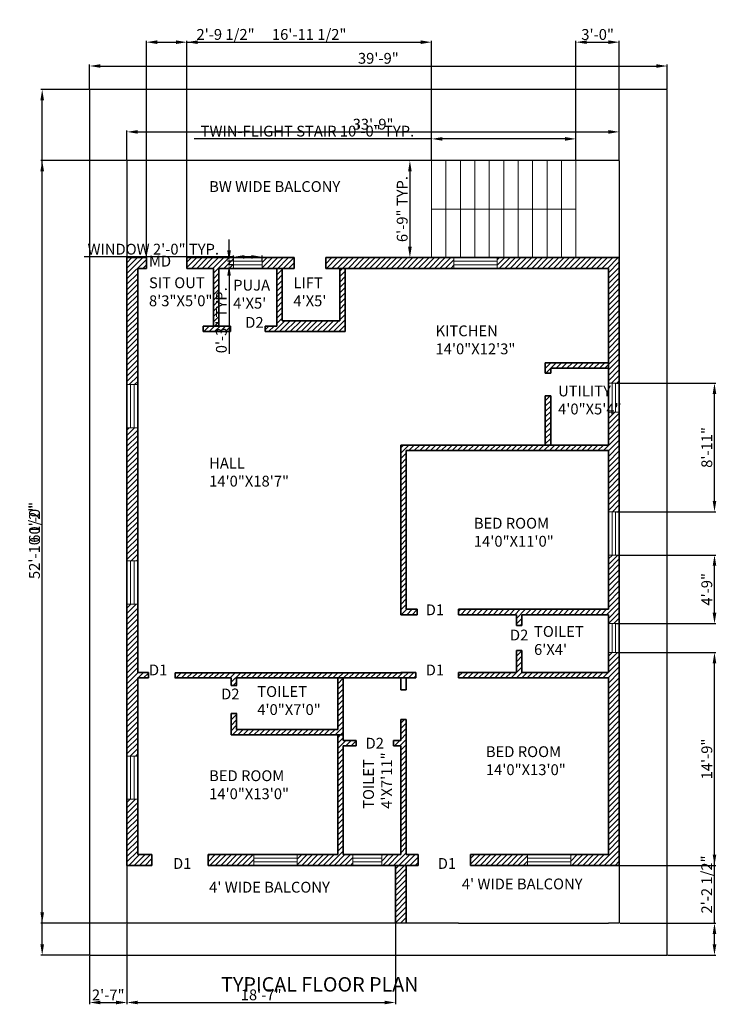
# Model space of a CAD drawing. Units: inches. Extents: x 9573 to 10767, y 4927 to 5746.
# Tile 2 of 2: x 10182 to 10767, y 4927 to 5746. Entities that reach past the tile are written whole.
import ezdxf

# ---------------------------------------------------------------- set-up
doc = ezdxf.new("R2010")
doc.units = ezdxf.units.IN
for name, color, linetype, lineweight in [('A-ANNO-DIMS', 2, 'Continuous', 18), ('A-ANNO-TEXT', 7, 'Continuous', 25), ('A-AREA-IDEN', 7, 'Continuous', 18), ('A-DOOR-IDEN', 3, 'Continuous', 18), ('A-FLOR-BALC', 7, 'Continuous', 25), ('A-FLOR-STRS', 7, 'Continuous', 18), ('A-GLAZ', 4, 'Continuous', 18), ('A-WALL', 7, 'Continuous', 35), ('A-WALL-PATT', 252, 'Continuous', 13), ('C-PROP', 8, 'Continuous', 25)]:
    doc.layers.add(name, color=color, linetype=linetype, lineweight=lineweight)
doc.styles.get("Standard").update_dxf_attribs({"font": 'arial.ttf'})
doc.dimstyles.new('ISO-25', dxfattribs={"dimtxt": 9, "dimasz": 9, "dimexe": 1.25, "dimexo": 0.625, "dimtad": 1, "dimdec": 1, "dimrnd": 9, "dimlunit": 3, "dimtxsty": 'Standard', "dimcen": 2.5, "dimadec": 0, "dimazin": 0, "dimtfac": 1, "dimtdec": 1, "dimtmove": 0, "dimatfit": 3, "dimfxl": 1, "dimarcsym": 0})
pattern_1 = [(45, (609.373, 0), (-2.245064, 2.245064), [])]

# ---------------------------------------------------------------- blocks, each defined once
blk = doc.blocks.new('*D3')
at = {"layer": 'A-ANNO-DIMS', "color": 0, "lineweight": -2, "transparency": 16777216}
for p, q in [((10271.02, 5629.81), (10271.02, 5654.25)), ((10280.02, 5653), (10671.21, 5653)), ((10680.21, 5629.81), (10680.21, 5654.25))]:
    blk.add_line(p, q, dxfattribs=at)
at = {"layer": 'A-ANNO-DIMS', "color": 0, "transparency": 16777216}
for points in [[(10280.02, 5654.5), (10280.02, 5651.5), (10271.02, 5653)], [(10671.21, 5654.5), (10671.21, 5651.5), (10680.21, 5653)]]:
    blk.add_solid(points, dxfattribs=at)
at = {"layer": 'Defpoints', "color": 0, "transparency": 16777216}
for p in [(10680.21, 5653), (10271.02, 5629.18), (10680.21, 5629.18)]:
    blk.add_point(p, dxfattribs=at)
at = {"layer": 'A-ANNO-DIMS', "color": 0, "transparency": 16777216, "insert": (10475.62, 5658.23), "char_height": 9, "attachment_point": 5}
blk.add_mtext('33\'-9"', dxfattribs=at)
blk = doc.blocks.new('*D4')
at = {"layer": 'A-ANNO-DIMS', "color": 0, "lineweight": -2, "transparency": 16777216}
for p, q in [((10240, 5688.89), (10240, 5709.04)), ((10249, 5707.79), (10711, 5707.79)), ((10720, 5688.89), (10720, 5709.04))]:
    blk.add_line(p, q, dxfattribs=at)
at = {"layer": 'A-ANNO-DIMS', "color": 0, "transparency": 16777216}
for points in [[(10249, 5709.29), (10249, 5706.29), (10240, 5707.79)], [(10711, 5709.29), (10711, 5706.29), (10720, 5707.79)]]:
    blk.add_solid(points, dxfattribs=at)
at = {"layer": 'Defpoints', "color": 0, "transparency": 16777216}
for p in [(10720, 5707.79), (10240, 5688.26), (10720, 5688.26)]:
    blk.add_point(p, dxfattribs=at)
at = {"layer": 'A-ANNO-DIMS', "color": 0, "transparency": 16777216, "insert": (10480, 5713.01), "char_height": 9, "attachment_point": 5}
blk.add_mtext('39\'-9"', dxfattribs=at)
blk = doc.blocks.new('GLAZ-36IN')
for p, q in [((0, 3), (36, 3)), ((0, 0), (36, 0))]:
    blk.add_line(p, q)
blk = doc.blocks.new('GLAZ-24IN')
for p, q in [((0, 3), (24, 3)), ((0, 0), (24, 0))]:
    blk.add_line(p, q)
blk = doc.blocks.new('STAIR-TWIN-FLIGHT')
for p, q in [((0, 80.77), (0, 0)), ((12, 80.77), (12, 0)), ((24, 80.77), (24, 0)), ((36, 80.77), (36, 0)), ((48, 80.77), (48, 0)), ((60, 80.77), (60, 0)), ((72, 80.77), (72, 0)), ((84, 80.77), (84, 0)), ((96, 80.77), (96, 0)), ((108, 80.77), (108, 0)), ((120, 80.77), (120, 0)), ((0, 40.39), (120, 40.39))]:
    blk.add_line(p, q)
blk = doc.blocks.new('*D10')
at = {"layer": 'A-ANNO-DIMS', "color": 0, "lineweight": -2, "transparency": 16777216}
for p, q in [((10359.53, 5549.01), (10235.39, 5549.01)), ((10359.53, 5546.03), (10359.53, 5550.26)), ((10374.53, 5549.01), (10368.53, 5549.01)), ((10383.53, 5546.03), (10383.53, 5550.26))]:
    blk.add_line(p, q, dxfattribs=at)
at = {"layer": 'A-ANNO-DIMS', "color": 0, "transparency": 16777216}
for points in [[(10368.53, 5550.51), (10368.53, 5547.51), (10359.53, 5549.01)], [(10374.53, 5550.51), (10374.53, 5547.51), (10383.53, 5549.01)]]:
    blk.add_solid(points, dxfattribs=at)
at = {"layer": 'Defpoints', "color": 0, "transparency": 16777216}
for p in [(10359.53, 5549.01), (10359.53, 5545.41), (10383.53, 5545.41)]:
    blk.add_point(p, dxfattribs=at)
at = {"layer": 'A-ANNO-DIMS', "color": 0, "transparency": 16777216, "insert": (10292.96, 5554.29), "char_height": 9, "attachment_point": 5}
blk.add_mtext('WINDOW 2\'-0" TYP.', dxfattribs=at)
blk = doc.blocks.new('*D11')
at = {"layer": 'A-ANNO-DIMS', "color": 0, "lineweight": -2, "transparency": 16777216}
for p, q in [((10355.93, 5554.41), (10355.93, 5563.41)), ((10358.9, 5545.41), (10354.68, 5545.41)), ((10355.93, 5545.41), (10355.93, 5542.41)), ((10358.9, 5542.41), (10354.68, 5542.41)), ((10355.93, 5533.41), (10355.93, 5468.3))]:
    blk.add_line(p, q, dxfattribs=at)
at = {"layer": 'A-ANNO-DIMS', "color": 0, "transparency": 16777216}
for points in [[(10354.43, 5554.41), (10357.43, 5554.41), (10355.93, 5545.41)], [(10354.43, 5533.41), (10357.43, 5533.41), (10355.93, 5542.41)]]:
    blk.add_solid(points, dxfattribs=at)
at = {"layer": 'Defpoints', "color": 0, "transparency": 16777216}
for p in [(10359.53, 5545.41), (10355.93, 5542.41), (10359.53, 5542.41)]:
    blk.add_point(p, dxfattribs=at)
at = {"layer": 'A-ANNO-DIMS', "color": 0, "transparency": 16777216, "insert": (10350.7, 5496.35), "char_height": 9, "attachment_point": 5, "rotation": 90}
blk.add_mtext('0\'-3" TYP.', dxfattribs=at)
blk = doc.blocks.new('*D12')
at = {"layer": 'A-ANNO-DIMS', "color": 0, "lineweight": -2, "transparency": 16777216}
for p, q in [((10524.21, 5647.18), (10326.86, 5647.18)), ((10524.21, 5629.81), (10524.21, 5648.43)), ((10635.21, 5647.18), (10533.21, 5647.18)), ((10644.21, 5629.81), (10644.21, 5648.43))]:
    blk.add_line(p, q, dxfattribs=at)
at = {"layer": 'A-ANNO-DIMS', "color": 0, "transparency": 16777216}
for points in [[(10533.21, 5648.68), (10533.21, 5645.68), (10524.21, 5647.18)], [(10635.21, 5648.68), (10635.21, 5645.68), (10644.21, 5647.18)]]:
    blk.add_solid(points, dxfattribs=at)
at = {"layer": 'Defpoints', "color": 0, "transparency": 16777216}
for p in [(10524.21, 5647.18), (10524.21, 5629.18), (10644.21, 5629.18)]:
    blk.add_point(p, dxfattribs=at)
at = {"layer": 'A-ANNO-DIMS', "color": 0, "transparency": 16777216, "insert": (10421.04, 5652.46), "char_height": 9, "attachment_point": 5}
blk.add_mtext('TWIN-FLIGHT STAIR 10\'-0" TYP.', dxfattribs=at)
blk = doc.blocks.new('*D13')
at = {"layer": 'A-ANNO-DIMS', "color": 0, "lineweight": -2, "transparency": 16777216}
for p, q in [((10523.59, 5629.18), (10504.96, 5629.18)), ((10506.21, 5620.18), (10506.21, 5557.41)), ((10523.59, 5548.41), (10504.96, 5548.41))]:
    blk.add_line(p, q, dxfattribs=at)
at = {"layer": 'A-ANNO-DIMS', "color": 0, "transparency": 16777216}
for points in [[(10504.71, 5620.18), (10507.71, 5620.18), (10506.21, 5629.18)], [(10504.71, 5557.41), (10507.71, 5557.41), (10506.21, 5548.41)]]:
    blk.add_solid(points, dxfattribs=at)
at = {"layer": 'Defpoints', "color": 0, "transparency": 16777216}
for p in [(10524.21, 5629.18), (10506.21, 5548.41), (10524.21, 5548.41)]:
    blk.add_point(p, dxfattribs=at)
at = {"layer": 'A-ANNO-DIMS', "color": 0, "transparency": 16777216, "insert": (10500.99, 5588.8), "char_height": 9, "attachment_point": 5, "rotation": 90}
blk.add_mtext('6\'-9" TYP.', dxfattribs=at)
blk = doc.blocks.new('*D18')
at = {"layer": 'A-ANNO-DIMS', "color": 0, "lineweight": -2, "transparency": 16777216}
for p, q in [((10270.39, 5629.18), (10199.4, 5629.18)), ((10200.65, 5003.91), (10200.65, 5620.18)), ((10270.39, 4994.91), (10199.4, 4994.91))]:
    blk.add_line(p, q, dxfattribs=at)
at = {"layer": 'A-ANNO-DIMS', "color": 0, "transparency": 16777216}
for points in [[(10199.15, 5620.18), (10202.15, 5620.18), (10200.65, 5629.18)], [(10199.15, 5003.91), (10202.15, 5003.91), (10200.65, 4994.91)]]:
    blk.add_solid(points, dxfattribs=at)
at = {"layer": 'Defpoints', "color": 0, "transparency": 16777216}
for p in [(10200.65, 5629.18), (10271.02, 5629.18), (10271.02, 4994.91)]:
    blk.add_point(p, dxfattribs=at)
at = {"layer": 'A-ANNO-DIMS', "color": 0, "transparency": 16777216, "insert": (10195.37, 5312.05), "char_height": 9, "attachment_point": 5, "rotation": 90}
blk.add_mtext('52\'-10 1/2"', dxfattribs=at)
blk = doc.blocks.new('*D19')
at = {"layer": 'A-ANNO-DIMS', "color": 0, "lineweight": -2, "transparency": 16777216}
for p, q in [((10239.38, 5688.26), (10199.4, 5688.26)), ((10200.65, 4977.26), (10200.65, 5679.26)), ((10239.38, 4968.26), (10199.4, 4968.26))]:
    blk.add_line(p, q, dxfattribs=at)
at = {"layer": 'A-ANNO-DIMS', "color": 0, "transparency": 16777216}
for points in [[(10199.15, 5679.26), (10202.15, 5679.26), (10200.65, 5688.26)], [(10199.15, 4977.26), (10202.15, 4977.26), (10200.65, 4968.26)]]:
    blk.add_solid(points, dxfattribs=at)
at = {"layer": 'Defpoints', "color": 0, "transparency": 16777216}
for p in [(10200.65, 5688.26), (10240, 5688.26), (10240, 4968.26)]:
    blk.add_point(p, dxfattribs=at)
at = {"layer": 'A-ANNO-DIMS', "color": 0, "transparency": 16777216, "insert": (10195.43, 5328.26), "char_height": 9, "attachment_point": 5, "rotation": 90}
blk.add_mtext('60\'-0"', dxfattribs=at)
blk = doc.blocks.new('*D20')
at = {"layer": 'A-ANNO-DIMS', "color": 0, "lineweight": -2, "transparency": 16777216}
for p, q in [((10271.02, 4994.28), (10271.02, 4927.66)), ((10240, 4967.64), (10240, 4927.66)), ((10249, 4928.91), (10262.02, 4928.91))]:
    blk.add_line(p, q, dxfattribs=at)
at = {"layer": 'A-ANNO-DIMS', "color": 0, "transparency": 16777216}
for points in [[(10249, 4930.41), (10249, 4927.41), (10240, 4928.91)], [(10262.02, 4930.41), (10262.02, 4927.41), (10271.02, 4928.91)]]:
    blk.add_solid(points, dxfattribs=at)
at = {"layer": 'Defpoints', "color": 0, "transparency": 16777216}
for p in [(10271.02, 4994.91), (10240, 4968.26), (10271.02, 4928.91)]:
    blk.add_point(p, dxfattribs=at)
at = {"layer": 'A-ANNO-DIMS', "color": 0, "transparency": 16777216, "insert": (10255.51, 4934.06), "char_height": 9, "attachment_point": 5}
blk.add_mtext('2\'-7"', dxfattribs=at)
blk = doc.blocks.new('*D21')
at = {"layer": 'A-ANNO-DIMS', "color": 0, "lineweight": -2, "transparency": 16777216}
for p, q in [((10759.35, 4994.91), (10759.35, 5050.21)), ((10680.84, 4994.91), (10760.6, 4994.91)), ((10759.35, 4977.26), (10759.35, 4985.91)), ((10720.62, 4968.26), (10760.6, 4968.26))]:
    blk.add_line(p, q, dxfattribs=at)
at = {"layer": 'A-ANNO-DIMS', "color": 0, "transparency": 16777216}
for points in [[(10757.85, 4985.91), (10760.85, 4985.91), (10759.35, 4994.91)], [(10757.85, 4977.26), (10760.85, 4977.26), (10759.35, 4968.26)]]:
    blk.add_solid(points, dxfattribs=at)
at = {"layer": 'Defpoints', "color": 0, "transparency": 16777216}
for p in [(10680.21, 4994.91), (10759.35, 4994.91), (10720, 4968.26)]:
    blk.add_point(p, dxfattribs=at)
at = {"layer": 'A-ANNO-DIMS', "color": 0, "transparency": 16777216, "insert": (10754.07, 5027.06), "char_height": 9, "attachment_point": 5, "rotation": 90}
blk.add_mtext('2\'-2 1/2"', dxfattribs=at)
blk = doc.blocks.new('*D23')
at = {"layer": 'A-ANNO-DIMS', "color": 0, "lineweight": -2, "transparency": 16777216}
for p, q in [((10644.21, 5629.81), (10644.21, 5728.86)), ((10653.21, 5727.61), (10671.21, 5727.61)), ((10680.21, 5629.81), (10680.21, 5728.86))]:
    blk.add_line(p, q, dxfattribs=at)
at = {"layer": 'A-ANNO-DIMS', "color": 0, "transparency": 16777216}
for points in [[(10653.21, 5729.11), (10653.21, 5726.11), (10644.21, 5727.61)], [(10671.21, 5729.11), (10671.21, 5726.11), (10680.21, 5727.61)]]:
    blk.add_solid(points, dxfattribs=at)
at = {"layer": 'Defpoints', "color": 0, "transparency": 16777216}
for p in [(10680.21, 5727.61), (10644.21, 5629.18), (10680.21, 5629.18)]:
    blk.add_point(p, dxfattribs=at)
at = {"layer": 'A-ANNO-DIMS', "color": 0, "transparency": 16777216, "insert": (10662.21, 5732.83), "char_height": 9, "attachment_point": 5}
blk.add_mtext('3\'-0"', dxfattribs=at)
blk = doc.blocks.new('*D26')
at = {"layer": 'A-ANNO-DIMS', "color": 0, "lineweight": -2, "transparency": 16777216}
for p, q in [((10287.2, 5549.03), (10287.2, 5728.86)), ((10296.2, 5727.61), (10311.84, 5727.61)), ((10320.84, 5549.03), (10320.84, 5728.86)), ((10320.84, 5727.61), (10376.14, 5727.61))]:
    blk.add_line(p, q, dxfattribs=at)
at = {"layer": 'A-ANNO-DIMS', "color": 0, "transparency": 16777216}
for points in [[(10296.2, 5729.11), (10296.2, 5726.11), (10287.2, 5727.61)], [(10311.84, 5729.11), (10311.84, 5726.11), (10320.84, 5727.61)]]:
    blk.add_solid(points, dxfattribs=at)
at = {"layer": 'Defpoints', "color": 0, "transparency": 16777216}
for p in [(10320.84, 5727.61), (10287.2, 5548.41), (10320.84, 5548.41)]:
    blk.add_point(p, dxfattribs=at)
at = {"layer": 'A-ANNO-DIMS', "color": 0, "transparency": 16777216, "insert": (10352.99, 5732.89), "char_height": 9, "attachment_point": 5}
blk.add_mtext('2\'-9 1/2"', dxfattribs=at)
blk = doc.blocks.new('*D27')
at = {"layer": 'A-ANNO-DIMS', "color": 0, "lineweight": -2, "transparency": 16777216}
for p, q in [((10320.84, 5549.03), (10320.84, 5728.86)), ((10329.84, 5727.61), (10515.21, 5727.61)), ((10524.21, 5629.81), (10524.21, 5728.86))]:
    blk.add_line(p, q, dxfattribs=at)
at = {"layer": 'A-ANNO-DIMS', "color": 0, "transparency": 16777216}
for points in [[(10329.84, 5729.11), (10329.84, 5726.11), (10320.84, 5727.61)], [(10515.21, 5729.11), (10515.21, 5726.11), (10524.21, 5727.61)]]:
    blk.add_solid(points, dxfattribs=at)
at = {"layer": 'Defpoints', "color": 0, "transparency": 16777216}
for p in [(10524.21, 5727.61), (10524.21, 5629.18), (10320.84, 5548.41)]:
    blk.add_point(p, dxfattribs=at)
at = {"layer": 'A-ANNO-DIMS', "color": 0, "transparency": 16777216, "insert": (10422.52, 5732.89), "char_height": 9, "attachment_point": 5}
blk.add_mtext('16\'-11 1/2"', dxfattribs=at)
blk = doc.blocks.new('*D31')
at = {"layer": 'A-ANNO-DIMS', "color": 0, "lineweight": -2, "transparency": 16777216}
for p, q in [((10677.84, 5220), (10760.6, 5220)), ((10759.35, 5051.91), (10759.35, 5211)), ((10680.84, 5042.91), (10760.6, 5042.91))]:
    blk.add_line(p, q, dxfattribs=at)
at = {"layer": 'A-ANNO-DIMS', "color": 0, "transparency": 16777216}
for points in [[(10757.85, 5211), (10760.85, 5211), (10759.35, 5220)], [(10757.85, 5051.91), (10760.85, 5051.91), (10759.35, 5042.91)]]:
    blk.add_solid(points, dxfattribs=at)
at = {"layer": 'Defpoints', "color": 0, "transparency": 16777216}
for p in [(10677.21, 5220), (10759.35, 5220), (10680.21, 5042.91)]:
    blk.add_point(p, dxfattribs=at)
at = {"layer": 'A-ANNO-DIMS', "color": 0, "transparency": 16777216, "insert": (10754.13, 5131.45), "char_height": 9, "attachment_point": 5, "rotation": 90}
blk.add_mtext('14\'-9"', dxfattribs=at)
blk = doc.blocks.new('*D32')
at = {"layer": 'A-ANNO-DIMS', "color": 0, "lineweight": -2, "transparency": 16777216}
for p, q in [((10677.84, 5301.09), (10760.6, 5301.09)), ((10759.35, 5253), (10759.35, 5292.09)), ((10677.84, 5244), (10760.6, 5244))]:
    blk.add_line(p, q, dxfattribs=at)
at = {"layer": 'A-ANNO-DIMS', "color": 0, "transparency": 16777216}
for points in [[(10757.85, 5292.09), (10760.85, 5292.09), (10759.35, 5301.09)], [(10757.85, 5253), (10760.85, 5253), (10759.35, 5244)]]:
    blk.add_solid(points, dxfattribs=at)
at = {"layer": 'Defpoints', "color": 0, "transparency": 16777216}
for p in [(10677.21, 5301.09), (10759.35, 5301.09), (10677.21, 5244)]:
    blk.add_point(p, dxfattribs=at)
at = {"layer": 'A-ANNO-DIMS', "color": 0, "transparency": 16777216, "insert": (10754.13, 5272.55), "char_height": 9, "attachment_point": 5, "rotation": 90}
blk.add_mtext('4\'-9"', dxfattribs=at)
blk = doc.blocks.new('*D33')
at = {"layer": 'A-ANNO-DIMS', "color": 0, "lineweight": -2, "transparency": 16777216}
for p, q in [((10677.84, 5444), (10760.6, 5444)), ((10759.35, 5346.09), (10759.35, 5435)), ((10677.84, 5337.09), (10760.6, 5337.09))]:
    blk.add_line(p, q, dxfattribs=at)
at = {"layer": 'A-ANNO-DIMS', "color": 0, "transparency": 16777216}
for points in [[(10757.85, 5435), (10760.85, 5435), (10759.35, 5444)], [(10757.85, 5346.09), (10760.85, 5346.09), (10759.35, 5337.09)]]:
    blk.add_solid(points, dxfattribs=at)
at = {"layer": 'Defpoints', "color": 0, "transparency": 16777216}
for p in [(10677.21, 5444), (10759.35, 5444), (10677.21, 5337.09)]:
    blk.add_point(p, dxfattribs=at)
at = {"layer": 'A-ANNO-DIMS', "color": 0, "transparency": 16777216, "insert": (10754.13, 5390.55), "char_height": 9, "attachment_point": 5, "rotation": 90}
blk.add_mtext('8\'-11"', dxfattribs=at)
blk = doc.blocks.new('*D35')
at = {"layer": 'A-ANNO-DIMS', "color": 0, "lineweight": -2, "transparency": 16777216}
for p, q in [((10271.02, 4994.28), (10271.02, 4927.66)), ((10494.21, 4994.28), (10494.21, 4927.66)), ((10280.02, 4928.91), (10485.21, 4928.91))]:
    blk.add_line(p, q, dxfattribs=at)
at = {"layer": 'A-ANNO-DIMS', "color": 0, "transparency": 16777216}
for points in [[(10280.02, 4930.41), (10280.02, 4927.41), (10271.02, 4928.91)], [(10485.21, 4930.41), (10485.21, 4927.41), (10494.21, 4928.91)]]:
    blk.add_solid(points, dxfattribs=at)
at = {"layer": 'Defpoints', "color": 0, "transparency": 16777216}
for p in [(10271.02, 4994.91), (10494.21, 4994.91), (10494.21, 4928.91)]:
    blk.add_point(p, dxfattribs=at)
at = {"layer": 'A-ANNO-DIMS', "color": 0, "transparency": 16777216, "insert": (10382.62, 4934.13), "char_height": 9, "attachment_point": 5}
blk.add_mtext('18\'-7"', dxfattribs=at)

msp = doc.modelspace()

# ---------------------------------------------------------------- hatches: boundary and pattern name
at = {"layer": 'A-WALL-PATT'}
h = msp.add_hatch(dxfattribs=at)
h.set_pattern_fill('ANSI31', color=256)
h.set_pattern_definition(pattern_1)
h.paths.add_polyline_path([(10409.99, 5548.41), (10383.53, 5548.41), (10383.53, 5539.41), (10409.99, 5539.41)])
h.paths.add_polyline_path([(10400.02, 5539.41), (10395.52, 5539.41), (10395.52, 5491.41), (10385.93, 5491.41), (10385.93, 5486.91), (10400.02, 5486.91), (10452.52, 5486.91), (10452.52, 5539.41), (10448.02, 5539.41), (10448.02, 5495.91), (10400.02, 5495.91)])
h.paths.add_polyline_path([(10357.22, 5491.41), (10334.5, 5491.41), (10334.5, 5486.91), (10357.22, 5486.91)])
h.paths.add_polyline_path([(10542.76, 5548.41), (10436.27, 5548.41), (10436.27, 5539.41), (10542.76, 5539.41)])
h.paths.add_polyline_path([(10680.21, 5548.41), (10578.76, 5548.41), (10578.76, 5539.41), (10671.21, 5539.41), (10671.21, 5444), (10680.21, 5444)])
h.paths.add_polyline_path([(10680.21, 5420), (10671.21, 5420), (10671.21, 5392.41), (10498.71, 5392.41), (10498.71, 5251.41), (10512.35, 5251.41), (10512.35, 5255.91), (10503.21, 5255.91), (10503.21, 5387.91), (10671.21, 5387.91), (10671.21, 5337.09), (10680.21, 5337.09)])
h.paths.add_polyline_path([(10623.21, 5433.61), (10618.71, 5433.61), (10618.71, 5392.41), (10623.21, 5392.41)])
h.paths.add_polyline_path([(10671.21, 5460.91), (10618.71, 5460.91), (10618.71, 5452.41), (10623.21, 5452.41), (10623.21, 5456.41), (10671.21, 5456.41)], flags=17)
h.paths.add_polyline_path([(10280.02, 5406.85), (10271.02, 5406.85), (10271.02, 5296.18), (10280.02, 5296.18)])
h.paths.add_polyline_path([(10280.02, 5486.91), (10280.02, 5491.41), (10280.02, 5539.41), (10287.2, 5539.41), (10287.2, 5548.41), (10271.02, 5548.41), (10271.02, 5442.85), (10280.02, 5442.85)])
h.paths.add_polyline_path([(10291.82, 5051.91), (10280.02, 5051.91), (10280.02, 5097.91), (10271.02, 5097.91), (10271.02, 5065.4), (10271.02, 5042.91), (10291.82, 5042.91)])
h.paths.add_polyline_path([(10450.71, 5198.91), (10446.21, 5198.91), (10446.21, 5155.91), (10362.21, 5155.91), (10362.21, 5169.21), (10357.71, 5169.21), (10357.71, 5151.41), (10450.71, 5151.41)])
h = msp.add_hatch(dxfattribs=at)
h.set_pattern_fill('ANSI31', color=256)
h.set_pattern_definition(pattern_1)
h.paths.add_polyline_path([(10376.44, 5051.91), (10338.48, 5051.91), (10338.48, 5042.91), (10376.44, 5042.91)])
h.paths.add_polyline_path([(10280.02, 5198.91), (10288.95, 5198.91), (10288.95, 5203.27), (10280.02, 5203.26), (10280.02, 5260.18), (10271.02, 5260.18), (10271.02, 5133.91), (10280.02, 5133.91)])
h.paths.add_polyline_path([(10458.85, 5051.91), (10450.71, 5051.91), (10450.71, 5142.41), (10461.55, 5142.41), (10461.55, 5146.91), (10450.71, 5146.91), (10450.71, 5151.41), (10446.21, 5151.41), (10446.21, 5051.91), (10412.44, 5051.91), (10412.44, 5042.91), (10458.85, 5042.91)])
h.paths.add_polyline_path([(10511.15, 5203.41), (10498.71, 5203.4), (10498.71, 5203.23), (10311.25, 5203.23), (10311.25, 5198.91), (10357.71, 5198.91), (10357.71, 5192.53), (10362.21, 5192.53), (10362.21, 5198.91), (10511.15, 5198.91)])
h.paths.add_polyline_path([(10503.21, 5164.29), (10498.71, 5164.29), (10498.71, 5146.91), (10492.55, 5146.91), (10492.55, 5142.41), (10498.71, 5142.41), (10498.71, 5051.91), (10482.85, 5051.91), (10482.85, 5042.91), (10512.97, 5042.91), (10512.97, 5051.91), (10503.21, 5051.91)])
h.paths.add_polyline_path([(10503.21, 5042.91), (10494.21, 5042.91), (10494.21, 4994.91), (10503.21, 4994.91)])
h.paths.add_polyline_path([(10603.97, 5051.91), (10556.66, 5051.91), (10556.66, 5042.91), (10603.97, 5042.91)], flags=17)
h.paths.add_polyline_path([(10680.21, 5065.4), (10680.21, 5220), (10671.21, 5220), (10671.21, 5203.41), (10599.21, 5203.41), (10599.21, 5221.8), (10594.71, 5221.8), (10594.71, 5203.41), (10546.72, 5203.41), (10546.72, 5198.91), (10671.21, 5198.91), (10671.21, 5051.91), (10639.97, 5051.91), (10639.97, 5042.91), (10671.21, 5042.91), (10680.21, 5042.91)])
h.paths.add_polyline_path([(10680.21, 5301.09), (10671.21, 5301.09), (10671.21, 5255.91), (10546.72, 5255.91), (10546.72, 5251.41), (10594.71, 5251.41), (10594.71, 5242.53), (10599.21, 5242.53), (10599.21, 5251.41), (10671.21, 5251.41), (10671.21, 5244), (10680.21, 5244)])
h.paths.add_polyline_path([(10359.53, 5548.41), (10320.84, 5548.41), (10320.84, 5539.41), (10343.02, 5539.41), (10343.02, 5491.41), (10347.52, 5491.41), (10347.52, 5539.41), (10359.53, 5539.41)])

# ---------------------------------------------------------------- linework, layer by layer
at = {"layer": 'A-FLOR-BALC'}
for p, q in [((10680.21, 5629.18), (10271.02, 5629.18)), ((10271.02, 5629.18), (10271.02, 5548.41)), ((10680.21, 5629.18), (10680.21, 5548.41)), ((10271.02, 5042.91), (10271.02, 4994.91)), ((10680.21, 5042.91), (10680.21, 4994.91)), ((10546.72, 4994.91), (10271.02, 4994.91)), ((10546.72, 4994.91), (10671.21, 4994.91)), ((10680.21, 4994.91), (10671.21, 4994.91))]:
    msp.add_line(p, q, dxfattribs=at)
at = {"layer": 'A-GLAZ'}
for p, q in [((10359.53, 5548.41), (10359.53, 5539.41)), ((10383.53, 5548.41), (10383.53, 5539.41)), ((10542.76, 5548.41), (10542.76, 5539.41)), ((10578.76, 5548.41), (10578.76, 5539.41)), ((10280.02, 5442.85), (10271.02, 5442.85)), ((10671.21, 5444), (10680.21, 5444)), ((10671.21, 5420), (10680.21, 5420)), ((10280.02, 5406.85), (10271.02, 5406.85)), ((10680.21, 5337.09), (10671.21, 5337.09)), ((10680.21, 5301.09), (10671.21, 5301.09)), ((10280.02, 5296.18), (10271.02, 5296.18)), ((10280.02, 5260.18), (10271.02, 5260.18)), ((10671.21, 5244), (10680.21, 5244)), ((10671.21, 5220), (10680.21, 5220)), ((10280.02, 5133.91), (10271.02, 5133.91)), ((10280.02, 5097.91), (10271.02, 5097.91)), ((10376.44, 5051.91), (10376.44, 5042.91)), ((10412.44, 5051.91), (10412.44, 5042.91)), ((10458.85, 5051.91), (10458.85, 5042.91)), ((10482.85, 5051.91), (10482.85, 5042.91)), ((10603.97, 5051.91), (10603.97, 5042.91)), ((10639.97, 5051.91), (10639.97, 5042.91))]:
    msp.add_line(p, q, dxfattribs=at)
at = {"layer": 'A-WALL'}
for p, q in [((10271.02, 5548.41), (10287.2, 5548.41)), ((10271.02, 5548.41), (10271.02, 5065.4)), ((10287.2, 5548.41), (10287.2, 5539.41)), ((10320.84, 5548.41), (10409.99, 5548.41)), ((10320.84, 5548.41), (10320.84, 5539.41)), ((10409.99, 5548.41), (10409.99, 5539.41)), ((10436.27, 5548.41), (10680.21, 5548.41)), ((10436.27, 5548.41), (10436.27, 5539.41)), ((10280.02, 5539.41), (10287.2, 5539.41)), ((10320.84, 5539.41), (10343.02, 5539.41)), ((10347.52, 5539.41), (10409.99, 5539.41)), ((10436.27, 5539.41), (10671.21, 5539.41)), ((10448.02, 5495.91), (10400.02, 5495.91)), ((10280.02, 5491.41), (10280.02, 5486.91)), ((10280.02, 5486.91), (10280.02, 5203.26)), ((10334.5, 5491.41), (10357.22, 5491.41)), ((10334.5, 5491.41), (10334.5, 5486.91)), ((10334.5, 5486.91), (10357.22, 5486.91)), ((10357.22, 5491.41), (10357.22, 5486.91)), ((10385.93, 5491.41), (10395.52, 5491.41)), ((10385.93, 5491.41), (10385.93, 5486.91)), ((10385.93, 5486.91), (10400.02, 5486.91)), ((10452.52, 5486.91), (10400.02, 5486.91)), ((10618.71, 5460.91), (10671.21, 5460.91)), ((10623.21, 5456.41), (10671.21, 5456.41)), ((10623.21, 5452.41), (10618.71, 5452.41)), ((10623.21, 5433.61), (10618.71, 5433.61)), ((10498.71, 5392.41), (10671.21, 5392.41)), ((10503.21, 5387.91), (10671.21, 5387.91)), ((10498.71, 5251.41), (10512.35, 5251.41)), ((10503.21, 5255.91), (10512.35, 5255.91)), ((10512.35, 5255.91), (10512.35, 5251.41)), ((10546.72, 5255.91), (10671.21, 5255.91)), ((10546.72, 5255.91), (10546.72, 5251.41)), ((10546.72, 5251.41), (10594.71, 5251.41)), ((10599.21, 5251.41), (10671.21, 5251.41)), ((10594.71, 5242.53), (10599.21, 5242.53)), ((10594.71, 5221.8), (10599.21, 5221.8)), ((10288.95, 5203.27), (10279.94, 5203.26)), ((10280.02, 5203.26), (10279.94, 5203.26)), ((10288.95, 5203.27), (10288.95, 5198.9)), ((10311.25, 5203.23), (10311.25, 5198.78)), ((10311.25, 5203.23), (10498.71, 5203.23)), ((10498.71, 5203.41), (10498.71, 5203.23)), ((10511.15, 5203.41), (10498.71, 5203.4)), ((10511.15, 5203.41), (10511.15, 5198.91)), ((10546.72, 5203.41), (10594.71, 5203.41)), ((10546.72, 5203.41), (10546.72, 5198.91)), ((10599.21, 5203.41), (10671.21, 5203.41)), ((10288.95, 5198.91), (10280.02, 5198.91)), ((10280.02, 5198.91), (10280.02, 5051.91)), ((10357.71, 5198.91), (10311.25, 5198.91)), ((10357.56, 5192.53), (10362.41, 5192.53)), ((10357.71, 5192.53), (10357.71, 5198.91)), ((10362.21, 5192.53), (10362.21, 5198.91)), ((10511.15, 5198.91), (10362.21, 5198.91)), ((10446.21, 5155.91), (10446.21, 5198.91)), ((10450.71, 5146.91), (10450.71, 5198.91)), ((10498.71, 5189.03), (10498.71, 5198.91)), ((10503.21, 5189.03), (10503.21, 5198.91)), ((10546.72, 5198.91), (10671.21, 5198.91)), ((10671.21, 5051.91), (10671.21, 5198.91)), ((10498.71, 5189.03), (10503.21, 5189.03)), ((10357.56, 5169.21), (10362.41, 5169.21)), ((10357.71, 5151.41), (10357.71, 5169.21)), ((10362.21, 5155.91), (10362.21, 5169.21)), ((10498.71, 5146.91), (10498.71, 5164.29)), ((10498.71, 5164.29), (10503.21, 5164.29)), ((10503.21, 5051.91), (10503.21, 5164.29)), ((10450.71, 5151.41), (10357.71, 5151.41)), ((10446.21, 5155.91), (10362.21, 5155.91)), ((10446.21, 5051.91), (10446.21, 5151.41)), ((10461.55, 5146.91), (10450.71, 5146.91)), ((10461.55, 5146.91), (10461.55, 5142.41)), ((10498.71, 5146.91), (10492.55, 5146.91)), ((10492.55, 5146.91), (10492.55, 5142.41)), ((10450.71, 5051.91), (10450.71, 5142.41)), ((10461.55, 5142.41), (10450.71, 5142.41)), ((10498.71, 5142.41), (10492.55, 5142.41)), ((10498.71, 5051.91), (10498.71, 5142.41)), ((10271.02, 5042.91), (10271.02, 5065.4)), ((10680.21, 5065.4), (10680.21, 5042.91)), ((10291.82, 5051.91), (10280.02, 5051.91)), ((10291.82, 5051.91), (10291.82, 5042.91)), ((10446.21, 5051.91), (10338.48, 5051.91)), ((10338.48, 5051.91), (10338.48, 5042.91)), ((10498.71, 5051.91), (10450.71, 5051.91)), ((10512.97, 5051.91), (10503.21, 5051.91)), ((10512.97, 5051.91), (10512.97, 5042.91)), ((10556.66, 5051.91), (10671.21, 5051.91)), ((10556.66, 5051.91), (10556.66, 5042.91)), ((10291.82, 5042.91), (10271.02, 5042.91)), ((10512.97, 5042.91), (10338.48, 5042.91)), ((10494.21, 4994.91), (10494.21, 5042.91)), ((10503.21, 4994.91), (10503.21, 5042.91)), ((10556.66, 5042.91), (10671.21, 5042.91)), ((10680.21, 5042.91), (10671.21, 5042.91))]:
    msp.add_line(p, q, dxfattribs=at)
for points in [[(10680.21, 5548.41), (10680.21, 5065.4)], [(10280.02, 5491.41), (10280.02, 5539.41)], [(10343.02, 5491.41), (10343.02, 5539.41)], [(10347.52, 5491.41), (10347.52, 5539.41)], [(10395.52, 5491.41), (10395.52, 5539.41)], [(10400.02, 5495.91), (10400.02, 5539.41)], [(10448.02, 5495.91), (10448.02, 5539.41)], [(10452.52, 5486.91), (10452.52, 5539.41)], [(10671.21, 5539.41), (10671.21, 5392.41)], [(10618.71, 5460.91), (10618.71, 5452.41)], [(10623.21, 5456.41), (10623.21, 5452.41)], [(10618.71, 5433.61), (10618.71, 5392.41)], [(10623.21, 5433.61), (10623.21, 5392.41)], [(10498.71, 5392.41), (10498.71, 5251.41)], [(10503.21, 5387.91), (10503.21, 5255.91)], [(10671.21, 5387.91), (10671.21, 5255.91)], [(10594.71, 5251.41), (10594.71, 5242.53)], [(10599.21, 5251.41), (10599.21, 5242.53)], [(10671.21, 5251.41), (10671.21, 5203.41)], [(10594.71, 5221.8), (10594.71, 5203.41)], [(10599.21, 5221.8), (10599.21, 5203.41)]]:
    msp.add_lwpolyline(points, dxfattribs=at)
at = {"layer": 'C-PROP'}
for p, q in [((10720, 5688.26), (10240, 5688.26)), ((10240, 5688.26), (10240, 4968.26)), ((10720, 4968.26), (10720, 5688.26)), ((10240, 4968.26), (10720, 4968.26))]:
    msp.add_line(p, q, dxfattribs=at)

# ---------------------------------------------------------------- block references
at = {"layer": 'A-FLOR-STRS', "rotation": 180}
msp.add_blockref('STAIR-TWIN-FLIGHT', (10644.21, 5629.18), dxfattribs=at)
at = {"layer": 'A-GLAZ'}
for name, p, rotation in [('GLAZ-24IN', (10383.53, 5545.41), 180), ('GLAZ-36IN', (10578.76, 5545.41), 180), ('GLAZ-36IN', (10277.02, 5406.85), 90.00000000000286), ('GLAZ-24IN', (10674.21, 5444), 270.0000000000043), ('GLAZ-36IN', (10677.21, 5301.09), 90.00000000000286), ('GLAZ-36IN', (10277.02, 5260.18), 90.0000000000031), ('GLAZ-24IN', (10674.21, 5244), 270.0000000000043), ('GLAZ-36IN', (10277.02, 5097.91), 90.00000000000266), ('GLAZ-36IN', (10412.44, 5048.91), 180), ('GLAZ-24IN', (10482.85, 5048.91), 180), ('GLAZ-36IN', (10639.97, 5048.91), 180)]:
    msp.add_blockref(name, p, dxfattribs=dict(at, rotation=rotation))

# ---------------------------------------------------------------- texts
at = {"layer": 'A-ANNO-TEXT', "insert": (10349.37, 4950), "char_height": 12, "attachment_point": 1}
msp.add_mtext_dynamic_manual_height_columns('TYPICAL FLOOR PLAN', width=390, gutter_width=12.5, heights=[0], dxfattribs=at)
at = {"layer": 'A-AREA-IDEN', "char_height": 2.5, "attachment_point": 1}
for s, insert in [('{\\H3.6x;BW WIDE BALCONY}', (10339.37, 5612.02)), ('{\\H3.6x;SIT OUT\\P8\'3"X5\'0"}', (10289.37, 5532.02)), ("{\\H3.6x;PUJA\\P4'X5'}", (10359.37, 5530)), ("{\\H3.6x;LIFT\\P4'X5'}", (10409.37, 5531.99)), ('{\\H3.6x;KITCHEN\\P14\'0"X12\'3"}', (10527.52, 5492.02)), ('{\\H3.6x;UTILITY\\P4\'0"X5\'4"}', (10629.37, 5442.02)), ('{\\H3.6x;HALL}\\P{\\H3.6x;14\'0"X18\'7"}', (10339.37, 5382.02)), ('{\\H3.6x;BED ROOM\\P14\'0"X11\'0"}', (10559.37, 5332.02)), ("{\\H3.6x;TOILET\\P6'X4'}", (10609.37, 5242.02)), ('{\\H3.6x;TOILET\\P4\'0"X7\'0"}', (10379.37, 5192.02)), ('{\\H3.6x;BED ROOM\\P14\'0"X13\'0"}', (10569.37, 5142.02)), ('{\\H3.6x;BED ROOM\\P14\'0"X13\'0"}', (10339.37, 5122.02)), ("{\\H3.6x;4' WIDE BALCONY}", (10339.37, 5029.31)), ("{\\H3.6x;4' WIDE BALCONY}", (10549.37, 5032.02))]:
    msp.add_mtext_dynamic_manual_height_columns(s, width=120, gutter_width=12.5, heights=[0], dxfattribs=dict(at, insert=insert))
at = {"layer": 'A-AREA-IDEN', "insert": (10467.34, 5090), "char_height": 2.5, "attachment_point": 1, "rotation": 90}
msp.add_mtext_dynamic_manual_height_columns('{\\H3.6x;TOILET\\P4\'X7\'11"}', width=120, gutter_width=12.5, heights=[0], dxfattribs=at)
at = {"layer": 'A-DOOR-IDEN', "char_height": 9, "attachment_point": 1}
for s, insert in [('MD', (10289.37, 5550)), ('D2', (10369.37, 5499.04)), ('D1', (10519.37, 5260)), ('D2', (10589.37, 5239.04)), ('D1', (10289.37, 5210)), ('D1', (10519.37, 5210)), ('D2', (10349.37, 5190)), ('D2', (10469.37, 5149.04)), ('D1', (10309.37, 5049.04)), ('D1', (10529.37, 5049.04))]:
    msp.add_mtext_dynamic_manual_height_columns(s, width=20, gutter_width=12.5, heights=[0], dxfattribs=dict(at, insert=insert))

# ---------------------------------------------------------------- dimensions: what is measured, and where the dimension line sits
at = {"layer": 'A-ANNO-DIMS'}
for base, p1, p2, override, picture, middle in [((10320.84, 5727.61), (10287.2, 5548.41), (10320.84, 5548.41), {"dimdec": 1, "dimlfac": 1, "dimrnd": 0, "dimzin": 1, "dimdsep": 46, "dimlunit": 4, "dimfrac": 2}, '*D26', (10352.99, 5732.89)), ((10524.21, 5727.61), (10320.84, 5548.41), (10524.21, 5629.18), {"dimdec": 1, "dimlfac": 1, "dimrnd": 0, "dimzin": 1, "dimdsep": 46, "dimlunit": 4, "dimfrac": 2}, '*D27', (10422.52, 5732.89)), ((10680.21, 5727.61), (10644.21, 5629.18), (10680.21, 5629.18), {"dimdec": 1, "dimlfac": 1, "dimrnd": 0, "dimzin": 1, "dimdsep": 46, "dimlunit": 4, "dimfrac": 2}, '*D23', (10662.21, 5732.83)), ((10720, 5707.79), (10240, 5688.26), (10720, 5688.26), {"dimclrd": 0, "dimclre": 0, "dimclrt": 0}, '*D4', (10480, 5713.01)), ((10680.21, 5653), (10271.02, 5629.18), (10680.21, 5629.18), {"dimclrd": 0, "dimclre": 0, "dimclrt": 0}, '*D3', (10475.62, 5658.23)), ((10271.02, 4928.91), (10240, 4968.26), (10271.02, 4994.91), {"dimdec": 1, "dimlfac": 1, "dimrnd": 0, "dimzin": 1, "dimdsep": 46, "dimlunit": 4, "dimfrac": 2}, '*D20', (10255.51, 4934.06)), ((10494.21, 4928.91), (10271.02, 4994.91), (10494.21, 4994.91), {"dimdec": 1, "dimlfac": 1, "dimrnd": 0, "dimzin": 1, "dimdsep": 46, "dimlunit": 4, "dimfrac": 2}, '*D35', (10382.62, 4934.13))]:
    dim = msp.add_linear_dim(base=base, p1=p1, p2=p2, dimstyle='ISO-25', override=override, dxfattribs=at)
    dim.commit()
    dim.dimension.update_dxf_attribs({"geometry": picture, "text_midpoint": middle})
for base, p1, p2, picture, middle in [((10200.65, 5688.26), (10240, 4968.26), (10240, 5688.26), '*D19', (10195.43, 5328.26)), ((10200.65, 5629.18), (10271.02, 4994.91), (10271.02, 5629.18), '*D18', (10195.37, 5312.05)), ((10759.35, 5444), (10677.21, 5337.09), (10677.21, 5444), '*D33', (10754.13, 5390.55)), ((10759.35, 5301.09), (10677.21, 5244), (10677.21, 5301.09), '*D32', (10754.13, 5272.55)), ((10759.35, 5220), (10680.21, 5042.91), (10677.21, 5220), '*D31', (10754.13, 5131.45)), ((10759.35, 4994.9089), (10720, 4968.2616), (10680.2123, 4994.9089), '*D21', (10754.0715, 5027.0584))]:
    dim = msp.add_linear_dim(base=base, p1=p1, p2=p2, angle=90, dimstyle='ISO-25', override={"dimdec": 1, "dimlfac": 1, "dimrnd": 0, "dimzin": 1, "dimdsep": 46, "dimlunit": 4, "dimfrac": 2}, dxfattribs=at)
    dim.commit()
    dim.dimension.update_dxf_attribs({"geometry": picture, "text_midpoint": middle})
for base, p1, p2, angle, text, picture, middle in [((10524.21, 5647.18), (10644.21, 5629.18), (10524.21, 5629.18), 180, 'TWIN-FLIGHT STAIR <> TYP.', '*D12', (10421.04, 5652.46)), ((10506.21, 5548.41), (10524.21, 5629.18), (10524.21, 5548.41), 270, '<> TYP.', '*D13', (10500.99, 5588.8)), ((10359.53, 5549.01), (10383.53, 5545.41), (10359.53, 5545.41), 180, 'WINDOW <> TYP.', '*D10', (10292.96, 5554.29)), ((10355.93, 5542.41), (10359.53, 5545.41), (10359.53, 5542.41), 270, '<> TYP.', '*D11', (10350.7, 5496.35))]:
    dim = msp.add_linear_dim(base=base, p1=p1, p2=p2, angle=angle, text=text, dimstyle='ISO-25', override={"dimdec": 1, "dimlfac": 1, "dimrnd": 0, "dimzin": 1, "dimdsep": 46, "dimlunit": 4, "dimfrac": 2}, dxfattribs=at)
    dim.commit()
    dim.dimension.update_dxf_attribs({"geometry": picture, "text_midpoint": middle})

doc.saveas('drawing.dxf')
